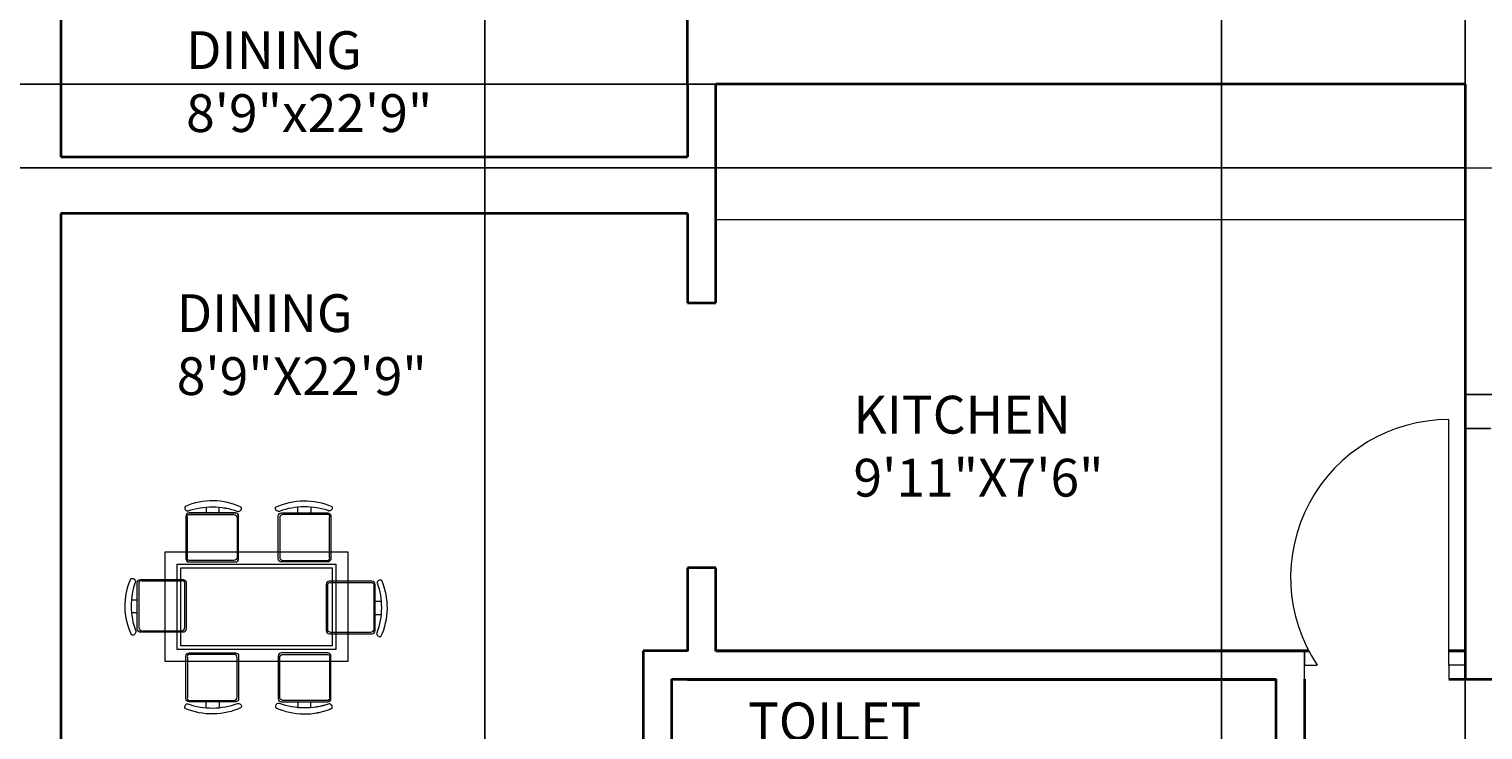
# Model space of a CAD drawing. Units: inches. Extents: x 1854 to 2495, y 1460 to 2772.
# Tile 5 of 12: x 2144 to 2375, y 1847 to 1958. Entities that reach past the tile are written whole.
import ezdxf

# ---------------------------------------------------------------- set-up
doc = ezdxf.new("R2010")
doc.units = ezdxf.units.IN
for name, color, linetype, lineweight in [('A-ANNO-DIMS', 2, 'Continuous', 18), ('A-AREA-IDEN', 7, 'Continuous', 18), ('A-DOOR', 3, 'Continuous', 18), ('A-FLOR-CASE', 8, 'Continuous', 18), ('A-FURN', 8, 'Continuous', 13), ('A-GLAZ', 4, 'Continuous', 18), ('A-WALL', 7, 'Continuous', 35)]:
    doc.layers.add(name, color=color, linetype=linetype, lineweight=lineweight)
doc.styles.get("Standard").update_dxf_attribs({"font": 'arial.ttf'})
doc.dimstyles.get("Standard").update_dxf_attribs({"dimtxt": 0.18, "dimasz": 0.18, "dimexe": 0.18, "dimexo": 0.0625, "dimgap": 0.09, "dimtad": 0, "dimtih": 1, "dimtoh": 1, "dimdec": 4, "dimzin": 0, "dimdsep": 46, "dimtxsty": 'Standard', "dimcen": 0.09, "dimadec": 0, "dimazin": 0, "dimtfac": 1, "dimtdec": 4, "dimtofl": 0, "dimtmove": 0, "dimatfit": 3, "dimfxl": 1, "dimtolj": 1, "dimtzin": 0, "dimarcsym": 0})

# ---------------------------------------------------------------- blocks, each defined once
blk = doc.blocks.new('WINDOW-36IN')
for p, q in [((0, 36), (9, 36)), ((9, 36), (4.5, 36)), ((4.5, 36), (4.5, 0)), ((4.5, 0), (0, 0)), ((0, 0), (9, 0))]:
    blk.add_line(p, q)
blk = doc.blocks.new('DINING-TABLE')
for points in [[(0, 17.41), (29.01, 17.41), (29.01, 0), (0, 0)], [(0, 17.41), (29.01, 17.41), (29.01, 0), (0, 0)], [(1.93, 15.47), (27.08, 15.47), (27.08, 1.93), (1.93, 1.93)], [(1.93, 15.47), (27.08, 15.47), (27.08, 1.93), (1.93, 1.93)], [(2.51, 14.89), (26.5, 14.89), (26.5, 2.51), (2.51, 2.51)], [(2.51, 14.89), (26.5, 14.89), (26.5, 2.51), (2.51, 2.51)]]:
    blk.add_lwpolyline(points, close=True)
blk = doc.blocks.new('DINING-CHAIR-END')
for points in [[(1.68, 0.62, -0.578392), (1.02, 0.02, -0.214524), (0.9, 8.94, -0.552014), (1.62, 8.53, 0.175809), (1.68, 0.62)], [(1.68, 0.62, -0.578392), (1.02, 0.02, -0.214524), (0.9, 8.94, -0.552014), (1.62, 8.52, 0.175809), (1.68, 0.62)], [(1.93, 8.29, -0.414214), (2.45, 8.81), (9.19, 8.81, -0.414214), (9.7, 8.29), (9.7, 0.96, -0.414214), (9.19, 0.45), (2.45, 0.45, -0.414214), (1.93, 0.96), (1.93, 8.29)], [(1.93, 8.29, -0.414214), (2.45, 8.81), (9.19, 8.81, -0.414214), (9.7, 8.29), (9.7, 0.96, -0.414214), (9.19, 0.45), (2.45, 0.45, -0.414214), (1.93, 0.96), (1.93, 8.29)], [(1.93, 3.54), (1, 3.54, 0.064759)], [(1.93, 3.54), (1, 3.54, 0.064759)]]:
    blk.add_lwpolyline(points, format="xyb")
blk.add_lwpolyline([(2.16, 8.29), (2.16, 1.19, 0.414214), (2.68, 0.68), (8.96, 0.68, 0.414214), (9.47, 1.19), (9.47, 8.29, 0.512069), (8.96, 8.58), (2.68, 8.58, 0.512069)], format="xyb", close=True)
blk.add_lwpolyline([(2.16, 8.29), (2.16, 1.19, 0.414214), (2.68, 0.68), (8.96, 0.68, 0.414214), (9.47, 1.19), (9.47, 8.29, 0.512069), (8.96, 8.58), (2.68, 8.58, 0.512069)], format="xyb", close=True)
blk.add_lwpolyline([(0.99, 5.59), (1.93, 5.59)])
blk.add_lwpolyline([(0.99, 5.59), (1.93, 5.59)])
blk = doc.blocks.new('DINING-CHAIR-01')
for points in [[(0.47, 8.09, -0.175809), (8.38, 8.03, 0.578392), (8.98, 8.69, 0.214524), (0.06, 8.81, 0.552014), (0.47, 8.09, -0.065079)], [(8.04, 7.77), (0.71, 7.77, 0.414214), (0.19, 7.26), (0.19, 0.51, 0.414214), (0.71, 0), (8.04, 0, 0.414214), (8.55, 0.51), (8.55, 7.26, 0.414214), (8.04, 7.77)], [(5.46, 7.77), (5.46, 8.7, -0.064759)]]:
    blk.add_lwpolyline(points, format="xyb")
blk.add_lwpolyline([(0.71, 7.54), (7.81, 7.54, -0.414214), (8.32, 7.03), (8.32, 0.74, -0.414214), (7.81, 0.23), (0.71, 0.23, -0.512069), (0.42, 0.74), (0.42, 7.03, -0.512069)], format="xyb", close=True)
blk.add_lwpolyline([(3.41, 8.72), (3.41, 7.77)])
blk = doc.blocks.new('DINING-CHAIR-06')
for points in [[(8.29, 1.93, 0.414214), (8.81, 2.45), (8.81, 9.19, 0.414214), (8.29, 9.7), (0.96, 9.7, 0.414214), (0.44, 9.19), (0.44, 2.45, 0.414214), (0.96, 1.93), (8.29, 1.93)], [(8.52, 1.62, -0.175809), (0.62, 1.68, 0.578392), (0.02, 1.02, 0.214524), (8.94, 0.9, 0.552014), (8.52, 1.62, -0.065079)], [(3.53, 1.93), (3.53, 1, -0.064759)]]:
    blk.add_lwpolyline(points, format="xyb")
blk.add_lwpolyline([(8.29, 2.16), (1.19, 2.16, -0.414214), (0.68, 2.68), (0.68, 8.96, -0.414214), (1.19, 9.47), (8.29, 9.47, -0.512069), (8.58, 8.96), (8.58, 2.68, -0.512069)], format="xyb", close=True)
blk.add_lwpolyline([(5.59, 0.99), (5.59, 1.93)])
blk = doc.blocks.new('*D26')
at = {"layer": 'A-ANNO-DIMS', "color": 0, "lineweight": -2, "transparency": 16777216}
for p, q in [((2371.98, 1899.73), (2371.98, 1894.21)), ((2380.98, 1899.73), (2380.98, 1894.21)), ((2372.16, 1894.39), (2376.02, 1894.39)), ((2380.8, 1894.39), (2376.94, 1894.39))]:
    blk.add_line(p, q, dxfattribs=at)
at = {"layer": 'A-ANNO-DIMS', "color": 0, "transparency": 16777216}
for points in [[(2372.16, 1894.42), (2372.16, 1894.36), (2371.98, 1894.39)], [(2380.8, 1894.42), (2380.8, 1894.36), (2380.98, 1894.39)]]:
    blk.add_solid(points, dxfattribs=at)
at = {"layer": 'Defpoints', "color": 0, "transparency": 16777216}
for p in [(2371.98, 1899.79), (2380.98, 1899.79), (2380.98, 1894.39)]:
    blk.add_point(p, dxfattribs=at)
at = {"layer": 'A-ANNO-DIMS', "color": 0, "transparency": 16777216, "insert": (2376.48, 1894.39), "char_height": 0.18, "attachment_point": 5}
blk.add_mtext('\\A1;9 TYP.', dxfattribs=at)
blk = doc.blocks.new('*D50')
at = {"layer": 'A-ANNO-DIMS', "color": 0, "lineweight": -2, "transparency": 16777216}
for p, q in [((2381.04, 2272.04), (2418.21, 2272.04)), ((2418.03, 2271.86), (2418.03, 1933.48)), ((2418.03, 1594.72), (2418.03, 1933.11)), ((2119.04, 1594.54), (2418.21, 1594.54))]:
    blk.add_line(p, q, dxfattribs=at)
at = {"layer": 'A-ANNO-DIMS', "color": 0, "transparency": 16777216}
for points in [[(2418, 2271.86), (2418.06, 2271.86), (2418.03, 2272.04)], [(2418, 1594.72), (2418.06, 1594.72), (2418.03, 1594.54)]]:
    blk.add_solid(points, dxfattribs=at)
at = {"layer": 'Defpoints', "color": 0, "transparency": 16777216}
for p in [(2380.98, 2272.04), (2418.03, 2272.04), (2118.98, 1594.54)]:
    blk.add_point(p, dxfattribs=at)
at = {"layer": 'A-ANNO-DIMS', "color": 0, "transparency": 16777216, "insert": (2418.03, 1933.29), "char_height": 0.18, "attachment_point": 5}
blk.add_mtext('\\A1;677.5', dxfattribs=at)
blk = doc.blocks.new('*D64')
at = {"layer": 'A-ANNO-DIMS', "color": 0, "lineweight": -2, "transparency": 16777216}
for p, q in [((2333.32, 2262.98), (2333.32, 1503.44)), ((2371.98, 2262.98), (2371.98, 1503.44)), ((2333.5, 1503.62), (2352.26, 1503.62)), ((2371.8, 1503.62), (2353.05, 1503.62))]:
    blk.add_line(p, q, dxfattribs=at)
at = {"layer": 'A-ANNO-DIMS', "color": 0, "transparency": 16777216}
for points in [[(2333.5, 1503.65), (2333.5, 1503.59), (2333.32, 1503.62)], [(2371.8, 1503.65), (2371.8, 1503.59), (2371.98, 1503.62)]]:
    blk.add_solid(points, dxfattribs=at)
at = {"layer": 'Defpoints', "color": 0, "transparency": 16777216}
for p in [(2333.32, 2263.04), (2371.98, 2263.04), (2371.98, 1503.62)]:
    blk.add_point(p, dxfattribs=at)
at = {"layer": 'A-ANNO-DIMS', "color": 0, "transparency": 16777216, "insert": (2352.65, 1503.62), "char_height": 0.18, "attachment_point": 5}
blk.add_mtext('\\A1;38.66', dxfattribs=at)
blk = doc.blocks.new('*D67')
at = {"layer": 'A-ANNO-DIMS', "color": 0, "lineweight": -2, "transparency": 16777216}
for p, q in [((2371.92, 1949.04), (1940.75, 1949.04)), ((1940.93, 1948.86), (1940.93, 1942.6)), ((1940.93, 1935.97), (1940.93, 1942.24)), ((2371.92, 1935.79), (1940.75, 1935.79))]:
    blk.add_line(p, q, dxfattribs=at)
at = {"layer": 'A-ANNO-DIMS', "color": 0, "transparency": 16777216}
for points in [[(1940.9, 1948.86), (1940.96, 1948.86), (1940.93, 1949.04)], [(1940.9, 1935.97), (1940.96, 1935.97), (1940.93, 1935.79)]]:
    blk.add_solid(points, dxfattribs=at)
at = {"layer": 'Defpoints', "color": 0, "transparency": 16777216}
for p in [(1940.93, 1949.04), (2371.98, 1949.04), (2371.98, 1935.79)]:
    blk.add_point(p, dxfattribs=at)
at = {"layer": 'A-ANNO-DIMS', "color": 0, "transparency": 16777216, "insert": (1940.93, 1942.42), "char_height": 0.18, "attachment_point": 5}
blk.add_mtext('\\A1;13.252', dxfattribs=at)
blk = doc.blocks.new('*D73')
at = {"layer": 'A-ANNO-DIMS', "color": 0, "lineweight": -2, "transparency": 16777216}
for p, q in [((2131.08, 2220.98), (2131.08, 1503.44)), ((2216.32, 2220.98), (2216.32, 1503.44)), ((2131.26, 1503.62), (2173.31, 1503.62)), ((2216.14, 1503.62), (2174.1, 1503.62))]:
    blk.add_line(p, q, dxfattribs=at)
at = {"layer": 'A-ANNO-DIMS', "color": 0, "transparency": 16777216}
for points in [[(2131.26, 1503.65), (2131.26, 1503.59), (2131.08, 1503.62)], [(2216.14, 1503.65), (2216.14, 1503.59), (2216.32, 1503.62)]]:
    blk.add_solid(points, dxfattribs=at)
at = {"layer": 'Defpoints', "color": 0, "transparency": 16777216}
for p in [(2131.08, 2221.04), (2216.32, 2221.04), (2216.32, 1503.62)]:
    blk.add_point(p, dxfattribs=at)
at = {"layer": 'A-ANNO-DIMS', "color": 0, "transparency": 16777216, "insert": (2173.7, 1503.62), "char_height": 0.18, "attachment_point": 5}
blk.add_mtext('\\A1;85.25', dxfattribs=at)

msp = doc.modelspace()

# ---------------------------------------------------------------- linework, layer by layer
at = {"layer": 'A-DOOR'}
for p, q in [((2369.391, 1856.8071), (2369.391, 1895.8071)), ((2346.4824, 1854.5571), (2346.4824, 1859.0571)), ((2346.4824, 1859.0571), (2346.4824, 1856.8071)), ((2346.4824, 1856.8071), (2348.4824, 1856.8071)), ((2371.9824, 1856.8071), (2369.391, 1856.8071)), ((2369.391, 1856.8071), (2369.391, 1854.5571))]:
    msp.add_line(p, q, dxfattribs=at)
msp.add_arc((2369.391, 1870.7024), 25.1047, 90, 213.606892, dxfattribs=at)
at = {"layer": 'A-FLOR-CASE'}
msp.add_line((2252.9824, 1927.5443), (2371.9824, 1927.5443), dxfattribs=at)
at = {"layer": 'A-FURN'}
for points in [[(2169.144, 1881.2816, -0.17580919), (2177.0457, 1881.2218, 0.57839206), (2177.6443, 1881.88, 0.21452438), (2168.725, 1881.9997, 0.55201397), (2169.144, 1881.2816, -0.06507904)], [(2174.1338, 1880.9645), (2174.1338, 1881.8922, -0.06475861)], [(2183.6979, 1881.2221, -0.57839206), (2183.0993, 1881.8803, -0.21452438), (2192.0186, 1882, -0.55201397), (2191.5996, 1881.2819, 0.1758092), (2183.6979, 1881.2221)], [(2183.6979, 1881.2218, -0.57839206), (2183.0993, 1881.88, -0.21452438), (2192.0187, 1881.9997, -0.55201397), (2191.5996, 1881.2816, 0.1758092), (2183.6979, 1881.2218)], [(2186.6098, 1880.9648), (2186.6098, 1881.8925, 0.06475861)], [(2186.6098, 1880.9645), (2186.6098, 1881.8922, 0.06475861)], [(2176.7105, 1880.9645), (2169.3748, 1880.9645, 0.41421356), (2168.8616, 1880.4512), (2168.8616, 1873.7062, 0.41421356), (2169.3748, 1873.193), (2176.7105, 1873.193, 0.41421356), (2177.2237, 1873.7062), (2177.2237, 1880.4512, 0.41421356), (2176.7105, 1880.9645)], [(2191.3688, 1880.9648, -0.41421356), (2191.882, 1880.4516), (2191.882, 1873.7065, -0.41421356), (2191.3688, 1873.1933), (2184.0331, 1873.1933, -0.41421356), (2183.5199, 1873.7065), (2183.5199, 1880.4516, -0.41421356), (2184.0331, 1880.9648), (2191.3688, 1880.9648)], [(2191.3688, 1880.9645, -0.41421356), (2191.882, 1880.4512), (2191.882, 1873.7062, -0.41421356), (2191.3688, 1873.193), (2184.0332, 1873.193, -0.41421356), (2183.52, 1873.7062), (2183.52, 1880.4512, -0.41421356), (2184.0332, 1880.9645), (2191.3688, 1880.9645)], [(2198.9099, 1869.6202, 0.41421356), (2198.3967, 1870.1334), (2191.6517, 1870.1334, 0.41421356), (2191.1384, 1869.6202), (2191.1384, 1862.2845, 0.41421356), (2191.6517, 1861.7713), (2198.3967, 1861.7713, 0.41421356), (2198.9099, 1862.2845), (2198.9099, 1869.6202)], [(2198.9099, 1869.6199, 0.41421356), (2198.3967, 1870.1331), (2191.6517, 1870.1331, 0.41421356), (2191.1385, 1869.6199), (2191.1385, 1862.2842, 0.41421356), (2191.6517, 1861.771), (2198.3967, 1861.771, 0.41421356), (2198.9099, 1862.2842), (2198.9099, 1869.6199)], [(2199.227, 1869.851, -0.17580919), (2199.1672, 1861.9493, 0.57839206), (2199.8254, 1861.3506, 0.21452438), (2199.9451, 1870.27, 0.55201397), (2199.227, 1869.851, -0.06507904)], [(2199.227, 1869.8507, -0.17580919), (2199.1672, 1861.949, 0.57839206), (2199.8254, 1861.3503, 0.21452438), (2199.9451, 1870.2697, 0.55201397), (2199.227, 1869.8507, -0.06507904)], [(2198.9099, 1864.8612), (2199.8376, 1864.8612, -0.06475861)], [(2198.9099, 1864.8608), (2199.8376, 1864.8608, -0.06475861)], [(2176.7105, 1850.9815), (2169.3748, 1850.9815, -0.41421356), (2168.8616, 1851.4948), (2168.8616, 1858.2398, -0.41421356), (2169.3748, 1858.753), (2176.7105, 1858.753, -0.41421356), (2177.2237, 1858.2398), (2177.2237, 1851.4948, -0.41421356), (2176.7105, 1850.9815)], [(2176.7105, 1850.9812), (2169.3748, 1850.9812, -0.41421356), (2168.8616, 1851.4945), (2168.8616, 1858.2395, -0.41421356), (2169.3748, 1858.7527), (2176.7105, 1858.7527, -0.41421356), (2177.2237, 1858.2395), (2177.2237, 1851.4945, -0.41421356), (2176.7105, 1850.9812)], [(2191.3688, 1850.9812, 0.41421356), (2191.882, 1851.4945), (2191.882, 1858.2395, 0.41421356), (2191.3688, 1858.7527), (2184.0332, 1858.7527, 0.41421356), (2183.52, 1858.2395), (2183.52, 1851.4945, 0.41421356), (2184.0332, 1850.9812), (2191.3688, 1850.9812)], [(2177.0457, 1850.7242, -0.57839206), (2177.6443, 1850.066, -0.21452438), (2168.725, 1849.9463, -0.55201397), (2169.144, 1850.6644, 0.17580929), (2177.0457, 1850.7242)], [(2177.0457, 1850.7239, -0.57839206), (2177.6443, 1850.0657, -0.21452438), (2168.725, 1849.946, -0.55201397), (2169.144, 1850.6641, 0.17580929), (2177.0457, 1850.7239)], [(2174.1338, 1850.9815), (2174.1338, 1850.0538, 0.06475861)], [(2174.1338, 1850.9812), (2174.1338, 1850.0535, 0.06475861)], [(2191.5996, 1850.6641, -0.17580928), (2183.6979, 1850.7239, 0.57839206), (2183.0993, 1850.0657, 0.21452438), (2192.0187, 1849.946, 0.55201397), (2191.5996, 1850.6641, -0.06507904)], [(2186.6098, 1850.9812), (2186.6098, 1850.0535, -0.06475861)]]:
    msp.add_lwpolyline(points, format="xyb", dxfattribs=at)
for points in [[(2172.0805, 1881.9091), (2172.0805, 1880.9645)], [(2188.6632, 1881.9094), (2188.6632, 1880.9648)], [(2188.6632, 1881.9091), (2188.6632, 1880.9645)], [(2199.8545, 1866.9145), (2198.9099, 1866.9145)], [(2199.8545, 1866.9142), (2198.9099, 1866.9142)], [(2172.0804, 1850.0369), (2172.0804, 1850.9815)], [(2172.0805, 1850.0366), (2172.0805, 1850.9812)], [(2188.6632, 1850.0366), (2188.6632, 1850.9812)]]:
    msp.add_lwpolyline(points, dxfattribs=at)
for points in [[(2169.3779, 1880.7333), (2176.4793, 1880.7333, -0.41421356), (2176.9925, 1880.22), (2176.9925, 1873.9374, -0.41421356), (2176.4793, 1873.4242), (2169.3779, 1873.4242, -0.51206948), (2169.0928, 1873.9374), (2169.0928, 1880.22, -0.51206948)], [(2191.3657, 1880.7336), (2184.2644, 1880.7336, 0.41421356), (2183.7511, 1880.2203), (2183.7511, 1873.9377, 0.41421356), (2184.2644, 1873.4245), (2191.3657, 1873.4245, 0.51206948), (2191.6508, 1873.9377), (2191.6508, 1880.2203, 0.51206948)], [(2191.3657, 1880.7333), (2184.2644, 1880.7333, 0.41421356), (2183.7512, 1880.22), (2183.7512, 1873.9374, 0.41421356), (2184.2644, 1873.4242), (2191.3657, 1873.4242, 0.51206948), (2191.6508, 1873.9374), (2191.6508, 1880.22, 0.51206948)], [(2198.6787, 1869.6171), (2198.6787, 1862.5157, -0.41421356), (2198.1655, 1862.0025), (2191.8829, 1862.0025, -0.41421356), (2191.3697, 1862.5157), (2191.3697, 1869.6171, -0.51206948), (2191.8829, 1869.9022), (2198.1655, 1869.9022, -0.51206948)], [(2198.6787, 1869.6168), (2198.6787, 1862.5154, -0.41421356), (2198.1655, 1862.0022), (2191.8829, 1862.0022, -0.41421356), (2191.3697, 1862.5154), (2191.3697, 1869.6168, -0.51206948), (2191.8829, 1869.9019), (2198.1655, 1869.9019, -0.51206948)], [(2169.3779, 1851.2127), (2176.4793, 1851.2127, 0.41421356), (2176.9925, 1851.726), (2176.9925, 1858.0086, 0.41421356), (2176.4793, 1858.5218), (2169.3779, 1858.5218, 0.51206948), (2169.0928, 1858.0086), (2169.0928, 1851.726, 0.51206948)], [(2169.3779, 1851.2124), (2176.4793, 1851.2124, 0.41421356), (2176.9925, 1851.7257), (2176.9925, 1858.0083, 0.41421356), (2176.4793, 1858.5215), (2169.3779, 1858.5215, 0.51206948), (2169.0928, 1858.0083), (2169.0928, 1851.7257, 0.51206948)], [(2191.3657, 1851.2124), (2184.2644, 1851.2124, -0.41421356), (2183.7512, 1851.7257), (2183.7512, 1858.0083, -0.41421356), (2184.2644, 1858.5215), (2191.3657, 1858.5215, -0.51206948), (2191.6508, 1858.0083), (2191.6508, 1851.7257, -0.51206948)]]:
    msp.add_lwpolyline(points, format="xyb", close=True, dxfattribs=at)
at = {"layer": 'A-WALL'}
for p, q in [((2148.9824, 2012.0449), (2148.9824, 1937.5287)), ((2248.4824, 1949.0449), (2248.4824, 1993.2912)), ((2248.4824, 1949.0449), (2248.4824, 1937.5287)), ((2371.9824, 1949.0449), (2252.9824, 1949.0449)), ((2252.9824, 1914.3387), (2252.9824, 1949.0449)), ((2371.9824, 1949.0449), (2371.9824, 1854.5571)), ((2371.9824, 1949.0449), (2371.9824, 1859.0449)), ((2148.9824, 1937.5287), (2248.4824, 1937.5287)), ((2248.4824, 1928.5287), (2148.9824, 1928.5287)), ((2148.9824, 1928.5287), (2148.9824, 1838.0449)), ((2248.4824, 1928.5287), (2248.4824, 1914.3387)), ((2248.4824, 1914.3387), (2252.9824, 1914.3387)), ((2252.9824, 1872.2802), (2248.4824, 1872.2802)), ((2248.4824, 1872.2802), (2248.4824, 1859.0449)), ((2248.4824, 1872.2802), (2248.4824, 1859.0571)), ((2252.9824, 1859.0449), (2252.9824, 1872.2802)), ((2252.9824, 1859.0571), (2252.9824, 1872.2802)), ((2241.4824, 1859.0571), (2241.4824, 1854.5571)), ((2248.4824, 1859.0571), (2241.4824, 1859.0571)), ((2241.4824, 1859.0571), (2241.4824, 1708.6844)), ((2347.1506, 1859.0571), (2252.9824, 1859.0571)), ((2347.157, 1859.0449), (2252.9824, 1859.0449)), ((2371.9824, 1859.0571), (2369.391, 1859.0571)), ((2371.9824, 1859.0449), (2369.391, 1859.0449)), ((2245.9824, 1854.5571), (2341.9824, 1854.5571)), ((2245.9824, 1854.5571), (2245.9824, 1800.5571)), ((2245.9824, 1854.5571), (2245.9824, 1800.5571)), ((2248.4824, 1854.5571), (2248.4824, 1854.5449)), ((2248.4824, 1854.5449), (2341.9824, 1854.5449)), ((2341.9824, 1800.5571), (2341.9824, 1854.5571)), ((2346.4824, 1854.5571), (2346.4824, 1800.5571)), ((2369.391, 1854.5571), (2380.9824, 1854.5571))]:
    msp.add_line(p, q, dxfattribs=at)

# ---------------------------------------------------------------- block references
at = {"layer": 'A-FURN'}
for name, p in [('DINING-CHAIR-01', (2168.6692, 1873.193)), ('DINING-CHAIR-END', (2159.2022, 1861.577)), ('DINING-CHAIR-06', (2183.0752, 1849.049))]:
    msp.add_blockref(name, p, dxfattribs=at)
at = {"layer": 'A-FURN', "rotation": 0.0007328377419428}
msp.add_blockref('DINING-TABLE', (2165.5553, 1857.3629), dxfattribs=at)
at = {"layer": 'A-GLAZ'}
msp.add_blockref('WINDOW-36IN', (2371.982, 1899.793), dxfattribs=at)

# ---------------------------------------------------------------- texts
at = {"layer": 'A-AREA-IDEN', "char_height": 6, "attachment_point": 1}
for s, width, insert in [('DINING\\P8\'9"x22\'9"', 73.191077, (2168.8765, 1957.4606)), ('DINING\\P8\'9"X22\'9"', 119.573347, (2167.3945, 1915.6973)), ('KITCHEN\\P9\'11"X7\'6"', 123.724846, (2274.8597, 1899.5745)), ('TOILET\\P8\'0"X4\'6"', 99.121381, (2258.1048, 1850.8764))]:
    msp.add_mtext_dynamic_manual_height_columns(s, width=width, gutter_width=12.5, heights=[0], dxfattribs=dict(at, insert=insert))

# ---------------------------------------------------------------- dimensions: what is measured, and where the dimension line sits
at = {"layer": 'A-ANNO-DIMS'}
for base, p1, p2, override, picture, middle in [((2418.0324, 2272.0449), (2118.9824, 1594.5449), (2380.9824, 2272.0449), {"dimdec": 1, "dimlfac": 1, "dimrnd": 0, "dimzin": 0, "dimdsep": 46, "dimlunit": 2}, '*D50', (2418.0324, 1933.2949)), ((1940.9324, 1949.0449), (2371.9824, 1935.7931), (2371.9824, 1949.0449), {"dimdec": 3, "dimlfac": 1, "dimrnd": 0, "dimzin": 0, "dimdsep": 46, "dimlunit": 2}, '*D67', (1940.9324, 1942.419))]:
    dim = msp.add_linear_dim(base=base, p1=p1, p2=p2, angle=90, dimstyle='Standard', override=override, dxfattribs=at)
    dim.commit()
    dim.dimension.update_dxf_attribs({"geometry": picture, "text_midpoint": middle})
for base, p1, p2, picture, middle in [((2371.9824, 1503.6207), (2333.3214, 2263.0449), (2371.9824, 2263.0449), '*D64', (2352.6519, 1503.6207)), ((2216.3239, 1503.6207), (2131.0775, 2221.0449), (2216.3239, 2221.0449), '*D73', (2173.7007, 1503.6207))]:
    dim = msp.add_linear_dim(base=base, p1=p1, p2=p2, dimstyle='Standard', override={"dimdec": 2, "dimlfac": 1, "dimrnd": 0, "dimzin": 0, "dimdsep": 46, "dimlunit": 2}, dxfattribs=at)
    dim.commit()
    dim.dimension.update_dxf_attribs({"geometry": picture, "text_midpoint": middle})
dim = msp.add_linear_dim(base=(2380.9824, 1894.3931), p1=(2371.9824, 1899.7931), p2=(2380.9824, 1899.7931), text='<> TYP.', dimstyle='Standard', override={"dimdec": 0, "dimlfac": 1, "dimrnd": 0, "dimzin": 0, "dimdsep": 46, "dimlunit": 2}, dxfattribs=at)
dim.commit()
dim.dimension.update_dxf_attribs({"geometry": '*D26', "text_midpoint": (2376.4824, 1894.3931)})

doc.saveas('drawing.dxf')
